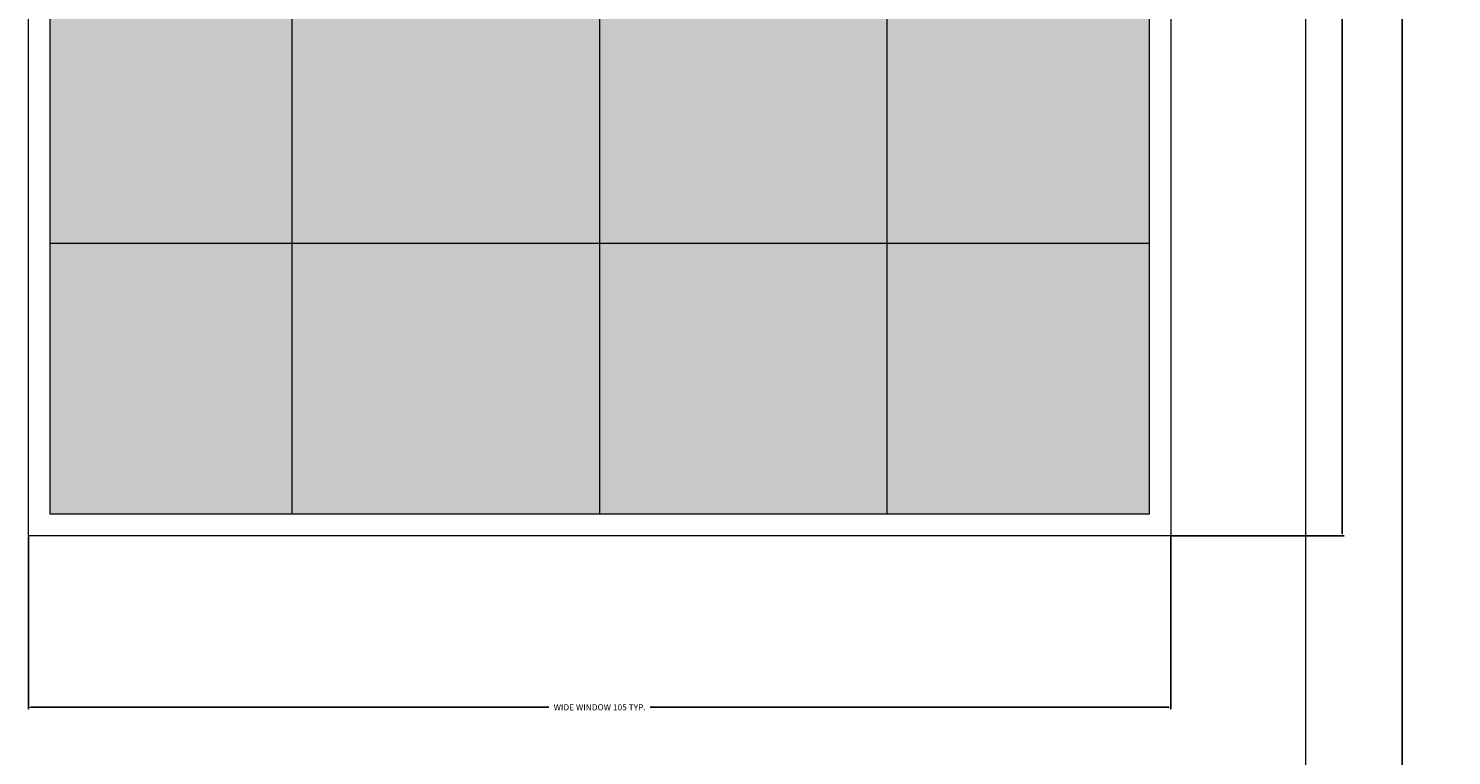
# Model space of a CAD drawing. Units: inches. Extents: x -26 to 776, y -22 to 650.
# Tile 12 of 62: x 92 to 222, y 287 to 353. Entities that reach past the tile are written whole.
import ezdxf

# ---------------------------------------------------------------- set-up
doc = ezdxf.new("R2010")
doc.units = ezdxf.units.IN
doc.header["$MEASUREMENT"] = 0
for name, color, linetype, lineweight in [('A-ANNO-DIMS', 2, 'Continuous', 18), ('A-GLAZ', 4, 'Continuous', 18), ('A-GLAZ-PATT', 9, 'Continuous', 13), ('A-WALL-TRIM', 7, 'Continuous', 18)]:
    doc.layers.add(name, color=color, linetype=linetype, lineweight=lineweight)
doc.styles.get("Standard").update_dxf_attribs({"font": 'arial.ttf'})
doc.dimstyles.get("Standard").update_dxf_attribs({"dimtxt": 0.5625, "dimasz": 0.18, "dimexe": 0.18, "dimexo": 0.0625, "dimgap": 0.09, "dimtad": 0, "dimtih": 1, "dimtoh": 1, "dimdec": 4, "dimzin": 0, "dimdsep": 46, "dimlunit": 4, "dimtxsty": 'Standard', "dimcen": 0.09, "dimadec": 0, "dimazin": 0, "dimtfac": 1, "dimtdec": 4, "dimtofl": 0, "dimtmove": 0, "dimatfit": 3, "dimfxl": 1, "dimtolj": 1, "dimtzin": 0, "dimarcsym": 0})

# ---------------------------------------------------------------- blocks, each defined once
blk = doc.blocks.new('WIN-ELEV-4X4')
for p, q in [((24.2, 97.34), (24.2, 2)), ((52.51, 97.34), (52.51, 2)), ((78.9, 97.34), (78.9, 2)), ((2, 76.47), (103.02, 76.47)), ((2, 76.47), (103.02, 76.47)), ((2, 52.37), (103.02, 52.37)), ((2, 26.9), (103.02, 26.9))]:
    blk.add_line(p, q)
for points in [[(0, 99.34), (105.02, 99.34), (105.02, 0), (0, 0)], [(2, 97.34), (103.02, 97.34), (103.02, 2), (2, 2)]]:
    blk.add_lwpolyline(points, close=True)
blk = doc.blocks.new('*D7')
at = {"layer": 'A-ANNO-DIMS', "color": 0, "lineweight": -2, "transparency": 16777216}
for p, q in [((91.64, 306.79), (91.64, 290.92)), ((196.67, 306.79), (196.67, 290.92)), ((91.82, 291.1), (139.5, 291.1)), ((196.49, 291.1), (148.81, 291.1))]:
    blk.add_line(p, q, dxfattribs=at)
at = {"layer": 'A-ANNO-DIMS', "color": 0, "transparency": 16777216}
for points in [[(91.82, 291.13), (91.82, 291.07), (91.64, 291.1)], [(196.49, 291.13), (196.49, 291.07), (196.67, 291.1)]]:
    blk.add_solid(points, dxfattribs=at)
at = {"layer": 'Defpoints', "color": 0, "transparency": 16777216}
for p in [(91.64, 306.86), (196.67, 306.86), (196.67, 291.1)]:
    blk.add_point(p, dxfattribs=at)
at = {"layer": 'A-ANNO-DIMS', "color": 0, "transparency": 16777216, "insert": (144.16, 291.1), "char_height": 0.5625, "attachment_point": 5}
blk.add_mtext('\\A1;WIDE WINDOW 105 TYP.', dxfattribs=at)
blk = doc.blocks.new('*D8')
at = {"layer": 'A-ANNO-DIMS', "color": 0, "lineweight": -2, "transparency": 16777216}
for p, q in [((196.73, 406.19), (212.6, 406.19)), ((212.42, 406.01), (212.42, 356.9)), ((212.42, 307.04), (212.42, 356.15)), ((196.73, 306.86), (212.6, 306.86))]:
    blk.add_line(p, q, dxfattribs=at)
at = {"layer": 'A-ANNO-DIMS', "color": 0, "transparency": 16777216}
for points in [[(212.39, 406.01), (212.45, 406.01), (212.42, 406.19)], [(212.39, 307.04), (212.45, 307.04), (212.42, 306.86)]]:
    blk.add_solid(points, dxfattribs=at)
at = {"layer": 'Defpoints', "color": 0, "transparency": 16777216}
for p in [(196.67, 406.19), (212.42, 406.19), (196.67, 306.86)]:
    blk.add_point(p, dxfattribs=at)
at = {"layer": 'A-ANNO-DIMS', "color": 0, "transparency": 16777216, "insert": (212.42, 356.52), "char_height": 0.5625, "attachment_point": 5}
blk.add_mtext('\\A1;99 TYP.', dxfattribs=at)
blk = doc.blocks.new('*D14')
at = {"layer": 'A-ANNO-DIMS', "color": 0, "lineweight": -2, "transparency": 16777216}
for p, q in [((191.62, 613.27), (-25.48, 613.27)), ((-25.3, 613.09), (-25.3, 314.75)), ((-25.3, 15.66), (-25.3, 314)), ((11.04, 15.48), (-25.48, 15.48))]:
    blk.add_line(p, q, dxfattribs=at)
at = {"layer": 'A-ANNO-DIMS', "color": 0, "transparency": 16777216}
for points in [[(-25.33, 613.09), (-25.27, 613.09), (-25.3, 613.27)], [(-25.33, 15.66), (-25.27, 15.66), (-25.3, 15.48)]]:
    blk.add_solid(points, dxfattribs=at)
at = {"layer": 'Defpoints', "color": 0, "transparency": 16777216}
for p in [(-25.3, 613.27), (191.68, 613.27), (11.11, 15.48)]:
    blk.add_point(p, dxfattribs=at)
at = {"layer": 'A-ANNO-DIMS', "color": 0, "transparency": 16777216, "insert": (-25.3, 314.38), "char_height": 0.562, "attachment_point": 5}
blk.add_mtext('\\A1;597.8', dxfattribs=at)
blk = doc.blocks.new('*D22')
at = {"layer": 'A-ANNO-DIMS', "color": 0, "lineweight": -2, "transparency": 16777216}
for p, q in [((22.89, 15.33), (22.89, 649.86)), ((23.07, 649.68), (119.19, 649.68)), ((217.77, 649.68), (121.65, 649.68)), ((217.95, 15.54), (217.95, 649.86))]:
    blk.add_line(p, q, dxfattribs=at)
at = {"layer": 'A-ANNO-DIMS', "color": 0, "transparency": 16777216}
for points in [[(23.07, 649.71), (23.07, 649.65), (22.89, 649.68)], [(217.77, 649.71), (217.77, 649.65), (217.95, 649.68)]]:
    blk.add_solid(points, dxfattribs=at)
at = {"layer": 'Defpoints', "color": 0, "transparency": 16777216}
for p in [(217.95, 649.68), (22.89, 15.27), (217.95, 15.48)]:
    blk.add_point(p, dxfattribs=at)
at = {"layer": 'A-ANNO-DIMS', "color": 0, "transparency": 16777216, "insert": (120.42, 649.68), "char_height": 0.562, "attachment_point": 5}
blk.add_mtext('\\A1;195.06', dxfattribs=at)

msp = doc.modelspace()

# ---------------------------------------------------------------- hatches: boundary and pattern name
at = {"layer": 'A-GLAZ-PATT'}
h = msp.add_hatch(dxfattribs=at)
h.set_pattern_fill('GOST_GLASS', color=256, scale=0.75)
h.set_pattern_definition([(45, (0, 0), (6.36396, 0), [3.75, -5.25]), (45, (1.591, 0), (6.36396, 0), [1.5, -7.5]), (45, (0, 1.591), (6.36396, 0), [1.5, -7.5])])
h.paths.add_polyline_path([(115.8402, 198.8773), (93.6448, 198.8773), (93.6448, 173.9734), (115.8402, 173.9734)])
h.paths.add_polyline_path([(144.1571, 198.8773), (115.8402, 198.8773), (115.8402, 173.9734), (144.1571, 173.9734)])
h.paths.add_polyline_path([(115.8402, 224.3396), (93.6448, 224.3396), (93.6448, 198.8773), (115.8402, 198.8773)])
h.paths.add_polyline_path([(144.1571, 248.4417), (115.8402, 248.4417), (115.8402, 224.3396), (144.1571, 224.3396)])
h.paths.add_polyline_path([(144.1571, 224.3396), (115.8402, 224.3396), (115.8402, 198.8773), (144.1571, 198.8773)])
h.paths.add_polyline_path([(170.5449, 224.3396), (144.1571, 224.3396), (144.1571, 198.8773), (170.5449, 198.8773)])
h.paths.add_polyline_path([(170.5449, 198.8773), (144.1571, 198.8773), (144.1571, 173.9734), (170.5449, 173.9734)])
h.paths.add_polyline_path([(194.6694, 198.8773), (170.5449, 198.8773), (170.5449, 173.9734), (194.6694, 173.9734)])
h.paths.add_polyline_path([(194.6694, 224.3396), (170.5449, 224.3396), (170.5449, 198.8773), (194.6694, 198.8773)])
h.paths.add_polyline_path([(194.6694, 248.4417), (170.5449, 248.4417), (170.5449, 224.3396), (194.6694, 224.3396)])
h.paths.add_polyline_path([(170.5449, 248.4417), (144.1571, 248.4417), (144.1571, 224.3396), (170.5449, 224.3396)])
h.paths.add_polyline_path([(144.1571, 269.3091), (115.8402, 269.3091), (115.8402, 248.4417), (144.1571, 248.4417)])
h.paths.add_polyline_path([(115.8402, 269.3091), (93.6448, 269.3091), (93.6448, 248.4417), (115.8402, 248.4417)])
h.paths.add_polyline_path([(115.8402, 248.4417), (93.6448, 248.4417), (93.6448, 224.3396), (115.8402, 224.3396)])
h.paths.add_polyline_path([(170.5449, 269.3091), (144.1571, 269.3091), (144.1571, 248.4417), (170.5449, 248.4417)])
h.paths.add_polyline_path([(194.6694, 269.3091), (170.5449, 269.3091), (170.5449, 248.4417), (194.6694, 248.4417)])
h.paths.add_polyline_path([(259.7413, 294.4171), (236.4647, 294.4171), (236.4647, 266.1888), (259.7413, 266.1888)])
h.paths.add_polyline_path([(285.0179, 294.4171), (261.7413, 294.4171), (261.7413, 266.1888), (285.0179, 266.1888)])
h.paths.add_polyline_path([(285.0179, 265.1888), (261.7413, 265.1888), (261.7413, 233.9172), (285.0179, 233.9172)])
h.paths.add_polyline_path([(259.7413, 265.1888), (236.4647, 265.1888), (236.4647, 233.9172), (259.7413, 233.9172)])
h.paths.add_polyline_path([(259.7413, 232.9172), (236.4647, 232.9172), (236.4647, 207.1741), (259.7413, 207.1741)])
h.paths.add_polyline_path([(285.0179, 232.9172), (261.7413, 232.9172), (261.7413, 207.1741), (285.0179, 207.1741)])
h.paths.add_polyline_path([(285.0179, 206.1741), (261.7413, 206.1741), (261.7413, 199.3298), (278.1134, 199.3298), (278.1134, 171.4173), (285.0179, 171.4173)])
h.paths.add_polyline_path([(259.7413, 206.1741), (236.4647, 206.1741), (236.4647, 199.3298), (259.7413, 199.3298)])
h.paths.add_polyline_path([(259.7413, 197.3298), (236.4647, 197.3298), (236.4647, 171.4173), (259.7413, 171.4173)])
h.paths.add_polyline_path([(276.1134, 197.3298), (261.7413, 197.3298), (261.7413, 171.4173), (276.1134, 171.4173)], flags=17)
h.paths.add_polyline_path([(255.8125, 548.0348), (228.5733, 548.0348), (228.5733, 528.3585), (255.8125, 528.3585)])
h.paths.add_polyline_path([(281.6181, 548.0348), (256.0792, 548.0348), (256.0792, 528.3585), (281.6181, 528.3585)])
h.paths.add_polyline_path([(308.8797, 548.0348), (281.789, 548.0348), (281.789, 528.3585), (308.8797, 528.3585)])
h.paths.add_polyline_path([(357.2724, 548.0995), (309.2457, 548.0348), (309.2457, 528.3585), (357.3034, 528.4233), (357.3034, 538.2614)])
h.paths.add_polyline_path([(259.7413, 437.1188), (236.4647, 437.1188), (236.4647, 408.8905), (259.7413, 408.8905)])
h.paths.add_polyline_path([(285.0179, 437.1188), (261.7413, 437.1188), (261.7413, 408.8905), (285.0179, 408.8905)])
h.paths.add_polyline_path([(259.7413, 407.8905), (236.4647, 407.8905), (236.4647, 376.6189), (259.7413, 376.6189)])
h.paths.add_polyline_path([(285.0179, 407.8905), (261.7413, 407.8905), (261.7413, 376.6189), (285.0179, 376.6189)])
h.paths.add_polyline_path([(285.0179, 375.6189), (261.7413, 375.6189), (261.7413, 349.8758), (285.0179, 349.8758)])
h.paths.add_polyline_path([(285.0179, 348.8758), (261.7413, 348.8758), (261.7413, 314.119), (285.0179, 314.119)])
h.paths.add_polyline_path([(259.7413, 348.8758), (236.4647, 348.8758), (236.4647, 314.119), (259.7413, 314.119)])
h.paths.add_polyline_path([(259.7413, 375.6189), (236.4647, 375.6189), (236.4647, 349.8758), (259.7413, 349.8758)])
h.paths.add_polyline_path([(194.6694, 404.1909), (170.5449, 404.1909), (170.5449, 383.3235), (194.6694, 383.3235)])
h.paths.add_polyline_path([(170.5449, 404.1909), (144.1571, 404.1909), (144.1571, 383.3235), (170.5449, 383.3235)])
h.paths.add_polyline_path([(144.1571, 404.1909), (115.8402, 404.1909), (115.8402, 383.3235), (144.1571, 383.3235)])
h.paths.add_polyline_path([(115.8402, 404.1909), (93.6448, 404.1909), (93.6448, 383.3235), (115.8402, 383.3235)])
h.paths.add_polyline_path([(115.8402, 383.3235), (93.6448, 383.3235), (93.6448, 359.2214), (115.8402, 359.2214)])
h.paths.add_polyline_path([(144.1571, 383.3235), (115.8402, 383.3235), (115.8402, 359.2214), (144.1571, 359.2214)])
h.paths.add_polyline_path([(115.8402, 359.2214), (93.6448, 359.2214), (93.6448, 333.7591), (115.8402, 333.7591)])
h.paths.add_polyline_path([(144.1571, 359.2214), (115.8402, 359.2214), (115.8402, 333.7591), (144.1571, 333.7591)])
h.paths.add_polyline_path([(115.8402, 333.7591), (93.6448, 333.7591), (93.6448, 308.8552), (115.8402, 308.8552)])
h.paths.add_polyline_path([(144.1571, 333.7591), (115.8402, 333.7591), (115.8402, 308.8552), (144.1571, 308.8552)])
h.paths.add_polyline_path([(170.5449, 333.7591), (144.1571, 333.7591), (144.1571, 308.8552), (170.5449, 308.8552)])
h.paths.add_polyline_path([(170.5449, 359.2214), (144.1571, 359.2214), (144.1571, 333.7591), (170.5449, 333.7591)])
h.paths.add_polyline_path([(170.5449, 383.3235), (144.1571, 383.3235), (144.1571, 359.2214), (170.5449, 359.2214)])
h.paths.add_polyline_path([(194.6694, 383.3235), (170.5449, 383.3235), (170.5449, 359.2214), (194.6694, 359.2214)])
h.paths.add_polyline_path([(194.6694, 359.2214), (170.5449, 359.2214), (170.5449, 333.7591), (194.6694, 333.7591)])
h.paths.add_polyline_path([(194.6694, 333.7591), (170.5449, 333.7591), (170.5449, 308.8552), (194.6694, 308.8552)])

# ---------------------------------------------------------------- linework, layer by layer
at = {"layer": 'A-WALL-TRIM'}
msp.add_lwpolyline([(82.134, 159.4824), (209.091, 159.4824), (209.091, 420.2783), (82.134, 420.2783)], close=True, dxfattribs=at)

# ---------------------------------------------------------------- block references
at = {"layer": 'A-GLAZ'}
msp.add_blockref('WIN-ELEV-4X4', (91.645, 306.855), dxfattribs=at)

# ---------------------------------------------------------------- dimensions: what is measured, and where the dimension line sits
at = {"layer": 'A-ANNO-DIMS'}
dim = msp.add_linear_dim(base=(217.9529, 649.6763), p1=(22.8891, 15.2701), p2=(217.9529, 15.4824), dimstyle='Standard', override={"dimdec": 2, "dimlfac": 1, "dimrnd": 0, "dimzin": 0, "dimdsep": 46, "dimlunit": 2}, dxfattribs=at)
dim.commit()
dim.dimension.update_dxf_attribs({"geometry": '*D22', "text_midpoint": (120.421, 649.6763)})
dim = msp.add_linear_dim(base=(-25.2976, 613.2713), p1=(11.1074, 15.4824), p2=(191.6782, 613.2713), angle=90, dimstyle='Standard', override={"dimdec": 1, "dimlfac": 1, "dimrnd": 0, "dimzin": 0, "dimdsep": 46, "dimlunit": 2}, dxfattribs=at)
dim.commit()
dim.dimension.update_dxf_attribs({"geometry": '*D14', "text_midpoint": (-25.2976, 314.3769)})
dim = msp.add_linear_dim(base=(212.4231, 406.1909), p1=(196.6694, 306.8552), p2=(196.6694, 406.1909), angle=90, text='<> TYP.', dimstyle='Standard', override={"dimdec": 0, "dimlfac": 1, "dimrnd": 0, "dimzin": 0, "dimdsep": 46, "dimlunit": 2}, dxfattribs=at)
dim.commit()
dim.dimension.update_dxf_attribs({"geometry": '*D8', "text_midpoint": (212.4231, 356.523)})
dim = msp.add_linear_dim(base=(196.6694, 291.1015), p1=(91.6448, 306.8552), p2=(196.6694, 306.8552), text='WIDE WINDOW <> TYP.', dimstyle='Standard', override={"dimdec": 0, "dimlfac": 1, "dimrnd": 0, "dimzin": 0, "dimdsep": 46, "dimlunit": 2}, dxfattribs=at)
dim.commit()
dim.dimension.update_dxf_attribs({"geometry": '*D7', "text_midpoint": (144.1571, 291.1015)})

doc.saveas('drawing.dxf')
